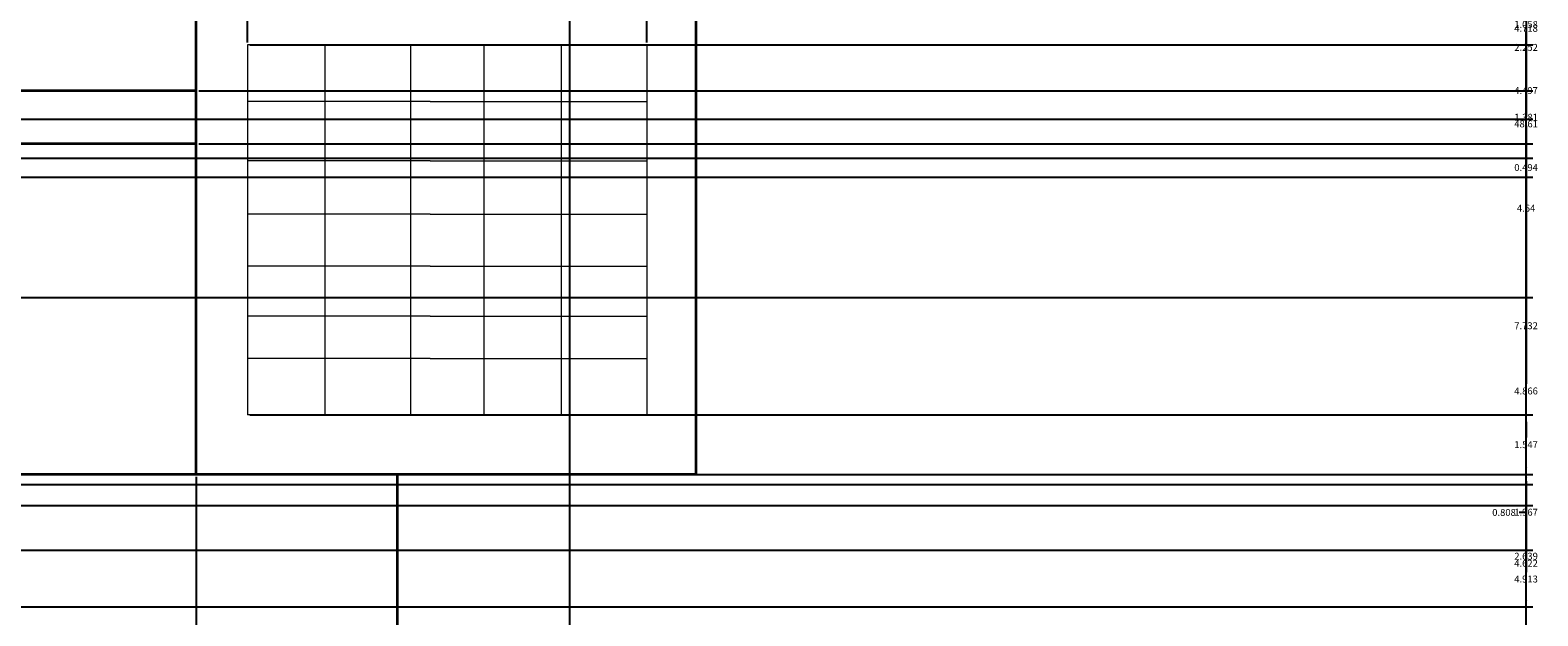
# Model space of a CAD drawing. Units: inches. Extents: x -10 to 130, y -32 to 34.
# Tile 20 of 22: x 90 to 130, y -10 to 5. Entities that reach past the tile are written whole.
import ezdxf

# ---------------------------------------------------------------- set-up
doc = ezdxf.new("R2010")
doc.units = ezdxf.units.IN
doc.header["$MEASUREMENT"] = 0
for name, color, linetype, lineweight in [('A-ANNO-DIMS', 2, 'Continuous', 18), ('A-ELEV', 7, 'Continuous', 35), ('A-GLAZ', 4, 'Continuous', 18)]:
    doc.layers.add(name, color=color, linetype=linetype, lineweight=lineweight)
doc.styles.get("Standard").update_dxf_attribs({"font": 'arial.ttf'})
doc.dimstyles.get("Standard").update_dxf_attribs({"dimtxt": 0.18, "dimasz": 0.18, "dimexe": 0.18, "dimexo": 0.0625, "dimgap": 0.09, "dimtad": 0, "dimtih": 1, "dimtoh": 1, "dimdec": 4, "dimzin": 0, "dimdsep": 46, "dimtxsty": 'Standard', "dimcen": 0.09, "dimadec": 0, "dimazin": 0, "dimtfac": 1, "dimtdec": 4, "dimtofl": 0, "dimtmove": 0, "dimatfit": 3, "dimfxl": 1, "dimtolj": 1, "dimtzin": 0, "dimarcsym": 0})

# ---------------------------------------------------------------- blocks, each defined once
blk = doc.blocks.new('*D2')
at = {"layer": 'A-ANNO-DIMS', "color": 0, "lineweight": -2, "transparency": 16777216}
for p, q in [((68.738, 27.199), (129.508, 27.199)), ((129.328, 27.019), (129.328, 3.074)), ((129.328, -21.234), (129.328, 2.71)), ((107.996, -21.414), (129.508, -21.414))]:
    blk.add_line(p, q, dxfattribs=at)
at = {"layer": 'A-ANNO-DIMS', "color": 0, "transparency": 16777216}
for points in [[(129.298, 27.019), (129.358, 27.019), (129.328, 27.199)], [(129.298, -21.234), (129.358, -21.234), (129.328, -21.414)]]:
    blk.add_solid(points, dxfattribs=at)
at = {"layer": 'Defpoints', "color": 0, "transparency": 16777216}
for p in [(68.676, 27.199), (129.328, 27.199), (107.933, -21.414)]:
    blk.add_point(p, dxfattribs=at)
at = {"layer": 'A-ANNO-DIMS', "color": 0, "transparency": 16777216, "insert": (129.328, 2.892), "char_height": 0.18, "attachment_point": 5}
blk.add_mtext('\\A1;48.61', dxfattribs=at)
blk = doc.blocks.new('*D66')
at = {"layer": 'A-ANNO-DIMS', "color": 0, "lineweight": -2, "transparency": 16777216}
for p, q in [((89.158, -16.844), (89.158, 33.879)), ((104.453, -13.219), (104.453, 33.879)), ((89.338, 33.699), (96.35, 33.699)), ((104.273, 33.699), (97.261, 33.699))]:
    blk.add_line(p, q, dxfattribs=at)
at = {"layer": 'A-ANNO-DIMS', "color": 0, "transparency": 16777216}
for points in [[(89.338, 33.729), (89.338, 33.669), (89.158, 33.699)], [(104.273, 33.729), (104.273, 33.669), (104.453, 33.699)]]:
    blk.add_solid(points, dxfattribs=at)
at = {"layer": 'Defpoints', "color": 0, "transparency": 16777216}
for p in [(104.453, 33.699), (104.453, -13.282), (89.158, -16.906)]:
    blk.add_point(p, dxfattribs=at)
at = {"layer": 'A-ANNO-DIMS', "color": 0, "transparency": 16777216, "insert": (96.805, 33.699), "char_height": 0.18, "attachment_point": 5}
blk.add_mtext('\\A1;15.295', dxfattribs=at)
blk = doc.blocks.new('*D76')
at = {"layer": 'A-ANNO-DIMS', "color": 0, "lineweight": -2, "transparency": 16777216}
for p, q in [((62.588, -6.485), (129.508, -6.485)), ((129.328, -6.665), (129.328, -8.76)), ((129.328, -11.218), (129.328, -9.123)), ((62.588, -11.398), (129.508, -11.398))]:
    blk.add_line(p, q, dxfattribs=at)
at = {"layer": 'A-ANNO-DIMS', "color": 0, "transparency": 16777216}
for points in [[(129.298, -6.665), (129.358, -6.665), (129.328, -6.485)], [(129.298, -11.218), (129.358, -11.218), (129.328, -11.398)]]:
    blk.add_solid(points, dxfattribs=at)
at = {"layer": 'Defpoints', "color": 0, "transparency": 16777216}
for p in [(62.526, -6.485), (129.328, -6.485), (62.526, -11.398)]:
    blk.add_point(p, dxfattribs=at)
at = {"layer": 'A-ANNO-DIMS', "color": 0, "transparency": 16777216, "insert": (129.328, -8.942), "char_height": 0.18, "attachment_point": 5}
blk.add_mtext('\\A1;4.913', dxfattribs=at)
blk = doc.blocks.new('*D77')
at = {"layer": 'A-ANNO-DIMS', "color": 0, "lineweight": -2, "transparency": 16777216}
for p, q in [((62.588, -1.618), (129.508, -1.618)), ((129.328, -1.798), (129.328, -3.87)), ((129.328, -6.305), (129.328, -4.234)), ((62.588, -6.485), (129.508, -6.485))]:
    blk.add_line(p, q, dxfattribs=at)
at = {"layer": 'A-ANNO-DIMS', "color": 0, "transparency": 16777216}
for points in [[(129.298, -1.798), (129.358, -1.798), (129.328, -1.618)], [(129.298, -6.305), (129.358, -6.305), (129.328, -6.485)]]:
    blk.add_solid(points, dxfattribs=at)
at = {"layer": 'Defpoints', "color": 0, "transparency": 16777216}
for p in [(62.526, -1.618), (129.328, -1.618), (62.526, -6.485)]:
    blk.add_point(p, dxfattribs=at)
at = {"layer": 'A-ANNO-DIMS', "color": 0, "transparency": 16777216, "insert": (129.328, -4.052), "char_height": 0.18, "attachment_point": 5}
blk.add_mtext('\\A1;4.866', dxfattribs=at)
blk = doc.blocks.new('*D78')
at = {"layer": 'A-ANNO-DIMS', "color": 0, "lineweight": -2, "transparency": 16777216}
for p, q in [((62.588, 3.018), (129.508, 3.018)), ((129.328, 2.838), (129.328, 0.882)), ((129.328, -1.438), (129.328, 0.518)), ((62.588, -1.618), (129.508, -1.618))]:
    blk.add_line(p, q, dxfattribs=at)
at = {"layer": 'A-ANNO-DIMS', "color": 0, "transparency": 16777216}
for points in [[(129.298, 2.838), (129.358, 2.838), (129.328, 3.018)], [(129.298, -1.438), (129.358, -1.438), (129.328, -1.618)]]:
    blk.add_solid(points, dxfattribs=at)
at = {"layer": 'Defpoints', "color": 0, "transparency": 16777216}
for p in [(62.526, 3.018), (129.328, 3.018), (62.526, -1.618)]:
    blk.add_point(p, dxfattribs=at)
at = {"layer": 'A-ANNO-DIMS', "color": 0, "transparency": 16777216, "insert": (129.328, 0.7), "char_height": 0.18, "attachment_point": 5}
blk.add_mtext('\\A1;4.64', dxfattribs=at)
blk = doc.blocks.new('*D79')
at = {"layer": 'A-ANNO-DIMS', "color": 0, "lineweight": -2, "transparency": 16777216}
for p, q in [((62.588, 7.736), (129.508, 7.736)), ((129.328, 7.556), (129.328, 5.559)), ((129.328, 3.198), (129.328, 5.195)), ((62.588, 3.018), (129.508, 3.018))]:
    blk.add_line(p, q, dxfattribs=at)
at = {"layer": 'A-ANNO-DIMS', "color": 0, "transparency": 16777216}
for points in [[(129.298, 7.556), (129.358, 7.556), (129.328, 7.736)], [(129.298, 3.198), (129.358, 3.198), (129.328, 3.018)]]:
    blk.add_solid(points, dxfattribs=at)
at = {"layer": 'Defpoints', "color": 0, "transparency": 16777216}
for p in [(62.526, 7.736), (129.328, 7.736), (62.526, 3.018)]:
    blk.add_point(p, dxfattribs=at)
at = {"layer": 'A-ANNO-DIMS', "color": 0, "transparency": 16777216, "insert": (129.328, 5.377), "char_height": 0.18, "attachment_point": 5}
blk.add_mtext('\\A1;4.718', dxfattribs=at)
blk = doc.blocks.new('*D153')
at = {"layer": 'A-ANNO-DIMS', "color": 0, "lineweight": -2, "transparency": 16777216}
for p, q in [((129.328, 2.185), (129.328, 2.365)), ((71.543, 2.005), (129.508, 2.005)), ((70.96, 1.511), (129.508, 1.511)), ((129.328, 1.331), (129.328, 1.151))]:
    blk.add_line(p, q, dxfattribs=at)
at = {"layer": 'A-ANNO-DIMS', "color": 0, "transparency": 16777216}
for points in [[(129.298, 2.185), (129.358, 2.185), (129.328, 2.005)], [(129.298, 1.331), (129.358, 1.331), (129.328, 1.511)]]:
    blk.add_solid(points, dxfattribs=at)
at = {"layer": 'Defpoints', "color": 0, "transparency": 16777216}
for p in [(71.48, 2.005), (70.898, 1.511), (129.328, 1.511)]:
    blk.add_point(p, dxfattribs=at)
at = {"layer": 'A-ANNO-DIMS', "color": 0, "transparency": 16777216, "insert": (129.328, 1.758), "char_height": 0.18, "attachment_point": 5}
blk.add_mtext('\\A1;0.494', dxfattribs=at)
blk = doc.blocks.new('*D154')
at = {"layer": 'A-ANNO-DIMS', "color": 0, "lineweight": -2, "transparency": 16777216}
for p, q in [((81.468, 6.007), (129.508, 6.007)), ((129.328, 5.827), (129.328, 3.941)), ((129.328, 1.691), (129.328, 3.577)), ((81.468, 1.511), (129.508, 1.511))]:
    blk.add_line(p, q, dxfattribs=at)
at = {"layer": 'A-ANNO-DIMS', "color": 0, "transparency": 16777216}
for points in [[(129.298, 5.827), (129.358, 5.827), (129.328, 6.007)], [(129.298, 1.691), (129.358, 1.691), (129.328, 1.511)]]:
    blk.add_solid(points, dxfattribs=at)
at = {"layer": 'Defpoints', "color": 0, "transparency": 16777216}
for p in [(81.405, 6.007), (129.328, 6.007), (81.405, 1.511)]:
    blk.add_point(p, dxfattribs=at)
at = {"layer": 'A-ANNO-DIMS', "color": 0, "transparency": 16777216, "insert": (129.328, 3.759), "char_height": 0.18, "attachment_point": 5}
blk.add_mtext('\\A1;4.497', dxfattribs=at)
blk = doc.blocks.new('*D159')
at = {"layer": 'A-ANNO-DIMS', "color": 0, "lineweight": -2, "transparency": 16777216}
for p, q in [((89.158, -6.284), (89.158, -28.129)), ((94.73, -6.284), (94.73, -28.129)), ((89.338, -27.949), (91.551, -27.949)), ((94.55, -27.949), (92.337, -27.949))]:
    blk.add_line(p, q, dxfattribs=at)
at = {"layer": 'A-ANNO-DIMS', "color": 0, "transparency": 16777216}
for points in [[(89.338, -27.919), (89.338, -27.979), (89.158, -27.949)], [(94.55, -27.919), (94.55, -27.979), (94.73, -27.949)]]:
    blk.add_solid(points, dxfattribs=at)
at = {"layer": 'Defpoints', "color": 0, "transparency": 16777216}
for p in [(89.158, -6.222), (94.73, -6.222), (94.73, -27.949)]:
    blk.add_point(p, dxfattribs=at)
at = {"layer": 'A-ANNO-DIMS', "color": 0, "transparency": 16777216, "insert": (91.944, -27.949), "char_height": 0.18, "attachment_point": 5}
blk.add_mtext('\\A1;5.572', dxfattribs=at)
blk = doc.blocks.new('*D160')
at = {"layer": 'A-ANNO-DIMS', "color": 0, "lineweight": -2, "transparency": 16777216}
for p, q in [((71.999, 1.511), (129.508, 1.511)), ((129.328, 1.331), (129.328, -2.174)), ((129.328, -6.042), (129.328, -2.538)), ((71.999, -6.222), (129.508, -6.222))]:
    blk.add_line(p, q, dxfattribs=at)
at = {"layer": 'A-ANNO-DIMS', "color": 0, "transparency": 16777216}
for points in [[(129.298, 1.331), (129.358, 1.331), (129.328, 1.511)], [(129.298, -6.042), (129.358, -6.042), (129.328, -6.222)]]:
    blk.add_solid(points, dxfattribs=at)
at = {"layer": 'Defpoints', "color": 0, "transparency": 16777216}
for p in [(71.937, 1.511), (71.937, -6.222), (129.328, -6.222)]:
    blk.add_point(p, dxfattribs=at)
at = {"layer": 'A-ANNO-DIMS', "color": 0, "transparency": 16777216, "insert": (129.328, -2.356), "char_height": 0.18, "attachment_point": 5}
blk.add_mtext('\\A1;7.732', dxfattribs=at)
blk = doc.blocks.new('*D161')
at = {"layer": 'A-ANNO-DIMS', "color": 0, "lineweight": -2, "transparency": 16777216}
for p, q in [((94.793, 6.007), (129.508, 6.007)), ((129.328, 5.827), (129.328, 5.064)), ((129.328, 3.936), (129.328, 4.7)), ((94.793, 3.756), (129.508, 3.756))]:
    blk.add_line(p, q, dxfattribs=at)
at = {"layer": 'A-ANNO-DIMS', "color": 0, "transparency": 16777216}
for points in [[(129.298, 5.827), (129.358, 5.827), (129.328, 6.007)], [(129.298, 3.936), (129.358, 3.936), (129.328, 3.756)]]:
    blk.add_solid(points, dxfattribs=at)
at = {"layer": 'Defpoints', "color": 0, "transparency": 16777216}
for p in [(94.73, 6.007), (94.73, 3.756), (129.328, 3.756)]:
    blk.add_point(p, dxfattribs=at)
at = {"layer": 'A-ANNO-DIMS', "color": 0, "transparency": 16777216, "insert": (129.328, 4.882), "char_height": 0.18, "attachment_point": 5}
blk.add_mtext('\\A1;2.252', dxfattribs=at)
blk = doc.blocks.new('*D162')
at = {"layer": 'A-ANNO-DIMS', "color": 0, "lineweight": -2, "transparency": 16777216}
for p, q in [((94.793, 3.756), (129.508, 3.756)), ((129.328, 3.576), (129.328, 3.247)), ((129.328, 2.555), (129.328, 2.883)), ((94.793, 2.375), (129.508, 2.375))]:
    blk.add_line(p, q, dxfattribs=at)
at = {"layer": 'A-ANNO-DIMS', "color": 0, "transparency": 16777216}
for points in [[(129.298, 3.576), (129.358, 3.576), (129.328, 3.756)], [(129.298, 2.555), (129.358, 2.555), (129.328, 2.375)]]:
    blk.add_solid(points, dxfattribs=at)
at = {"layer": 'Defpoints', "color": 0, "transparency": 16777216}
for p in [(94.73, 3.756), (94.73, 2.375), (129.328, 2.375)]:
    blk.add_point(p, dxfattribs=at)
at = {"layer": 'A-ANNO-DIMS', "color": 0, "transparency": 16777216, "insert": (129.328, 3.065), "char_height": 0.18, "attachment_point": 5}
blk.add_mtext('\\A1;1.381', dxfattribs=at)
blk = doc.blocks.new('*D163')
at = {"layer": 'A-ANNO-DIMS', "color": 0, "lineweight": -2, "transparency": 16777216}
for p, q in [((94.73, 6.07), (94.73, 33.879)), ((96.061, 5.012), (96.061, 33.879)), ((94.91, 33.699), (95.01, 33.699)), ((95.881, 33.699), (95.78, 33.699))]:
    blk.add_line(p, q, dxfattribs=at)
at = {"layer": 'A-ANNO-DIMS', "color": 0, "transparency": 16777216}
for points in [[(94.91, 33.729), (94.91, 33.669), (94.73, 33.699)], [(95.881, 33.729), (95.881, 33.669), (96.061, 33.699)]]:
    blk.add_solid(points, dxfattribs=at)
at = {"layer": 'Defpoints', "color": 0, "transparency": 16777216}
for p in [(96.061, 33.699), (94.73, 6.007), (96.061, 4.95)]:
    blk.add_point(p, dxfattribs=at)
at = {"layer": 'A-ANNO-DIMS', "color": 0, "transparency": 16777216, "insert": (95.395, 33.699), "char_height": 0.18, "attachment_point": 5}
blk.add_mtext('\\A1;1.330', dxfattribs=at)
blk = doc.blocks.new('*D164')
at = {"layer": 'A-ANNO-DIMS', "color": 0, "lineweight": -2, "transparency": 16777216}
for p, q in [((96.061, 5.012), (96.061, 33.879)), ((106.454, 5.012), (106.454, 33.879)), ((96.241, 33.699), (100.803, 33.699)), ((106.274, 33.699), (101.712, 33.699))]:
    blk.add_line(p, q, dxfattribs=at)
at = {"layer": 'A-ANNO-DIMS', "color": 0, "transparency": 16777216}
for points in [[(96.241, 33.729), (96.241, 33.669), (96.061, 33.699)], [(106.274, 33.729), (106.274, 33.669), (106.454, 33.699)]]:
    blk.add_solid(points, dxfattribs=at)
at = {"layer": 'Defpoints', "color": 0, "transparency": 16777216}
for p in [(106.454, 33.699), (96.061, 4.95), (106.454, 4.95)]:
    blk.add_point(p, dxfattribs=at)
at = {"layer": 'A-ANNO-DIMS', "color": 0, "transparency": 16777216, "insert": (101.257, 33.699), "char_height": 0.18, "attachment_point": 5}
blk.add_mtext('\\A1;10.394', dxfattribs=at)
blk = doc.blocks.new('*D165')
at = {"layer": 'A-ANNO-DIMS', "color": 0, "lineweight": -2, "transparency": 16777216}
for p, q in [((94.793, 6.007), (129.508, 6.007)), ((129.328, 5.827), (129.328, 5.66)), ((129.328, 5.13), (129.328, 5.297)), ((96.123, 4.95), (129.508, 4.95))]:
    blk.add_line(p, q, dxfattribs=at)
at = {"layer": 'A-ANNO-DIMS', "color": 0, "transparency": 16777216}
for points in [[(129.298, 5.827), (129.358, 5.827), (129.328, 6.007)], [(129.298, 5.13), (129.358, 5.13), (129.328, 4.95)]]:
    blk.add_solid(points, dxfattribs=at)
at = {"layer": 'Defpoints', "color": 0, "transparency": 16777216}
for p in [(94.73, 6.007), (129.328, 6.007), (96.061, 4.95)]:
    blk.add_point(p, dxfattribs=at)
at = {"layer": 'A-ANNO-DIMS', "color": 0, "transparency": 16777216, "insert": (129.328, 5.478), "char_height": 0.18, "attachment_point": 5}
blk.add_mtext('\\A1;1.058', dxfattribs=at)
blk = doc.blocks.new('*D166')
at = {"layer": 'A-ANNO-DIMS', "color": 0, "lineweight": -2, "transparency": 16777216}
for p, q in [((96.123, -4.675), (129.508, -4.675)), ((129.328, -4.855), (129.328, -5.266)), ((129.328, -6.042), (129.328, -5.63)), ((94.793, -6.222), (129.508, -6.222))]:
    blk.add_line(p, q, dxfattribs=at)
at = {"layer": 'A-ANNO-DIMS', "color": 0, "transparency": 16777216}
for points in [[(129.298, -4.855), (129.358, -4.855), (129.328, -4.675)], [(129.298, -6.042), (129.358, -6.042), (129.328, -6.222)]]:
    blk.add_solid(points, dxfattribs=at)
at = {"layer": 'Defpoints', "color": 0, "transparency": 16777216}
for p in [(96.061, -4.675), (94.73, -6.222), (129.328, -6.222)]:
    blk.add_point(p, dxfattribs=at)
at = {"layer": 'A-ANNO-DIMS', "color": 0, "transparency": 16777216, "insert": (129.328, -5.448), "char_height": 0.18, "attachment_point": 5}
blk.add_mtext('\\A1;1.547', dxfattribs=at)
blk = doc.blocks.new('*D168')
at = {"layer": 'A-ANNO-DIMS', "color": 0, "lineweight": -2, "transparency": 16777216}
for p, q in [((71.999, -6.222), (129.508, -6.222)), ((129.328, -6.402), (129.328, -7.024)), ((129.328, -8.009), (129.328, -7.387)), ((71.999, -8.189), (129.508, -8.189))]:
    blk.add_line(p, q, dxfattribs=at)
at = {"layer": 'A-ANNO-DIMS', "color": 0, "transparency": 16777216}
for points in [[(129.298, -6.402), (129.358, -6.402), (129.328, -6.222)], [(129.298, -8.009), (129.358, -8.009), (129.328, -8.189)]]:
    blk.add_solid(points, dxfattribs=at)
at = {"layer": 'Defpoints', "color": 0, "transparency": 16777216}
for p in [(71.937, -6.222), (71.937, -8.189), (129.328, -8.189)]:
    blk.add_point(p, dxfattribs=at)
at = {"layer": 'A-ANNO-DIMS', "color": 0, "transparency": 16777216, "insert": (129.328, -7.205), "char_height": 0.18, "attachment_point": 5}
blk.add_mtext('\\A1;1.967', dxfattribs=at)
blk = doc.blocks.new('*D171')
at = {"layer": 'A-ANNO-DIMS', "color": 0, "lineweight": -2, "transparency": 16777216}
for p, q in [((79.602, -7.03), (129.508, -7.03)), ((129.328, -7.21), (129.328, -8.167)), ((129.328, -9.489), (129.328, -8.531)), ((79.602, -9.669), (129.508, -9.669))]:
    blk.add_line(p, q, dxfattribs=at)
at = {"layer": 'A-ANNO-DIMS', "color": 0, "transparency": 16777216}
for points in [[(129.298, -7.21), (129.358, -7.21), (129.328, -7.03)], [(129.298, -9.489), (129.358, -9.489), (129.328, -9.669)]]:
    blk.add_solid(points, dxfattribs=at)
at = {"layer": 'Defpoints', "color": 0, "transparency": 16777216}
for p in [(79.539, -7.03), (79.539, -9.669), (129.328, -9.669)]:
    blk.add_point(p, dxfattribs=at)
at = {"layer": 'A-ANNO-DIMS', "color": 0, "transparency": 16777216, "insert": (129.328, -8.349), "char_height": 0.18, "attachment_point": 5}
blk.add_mtext('\\A1;2.639', dxfattribs=at)
blk = doc.blocks.new('*D172')
at = {"layer": 'A-ANNO-DIMS', "color": 0, "lineweight": -2, "transparency": 16777216}
for p, q in [((89.22, -6.222), (129.508, -6.222)), ((129.328, -6.402), (129.328, -6.85)), ((88.064, -7.03), (129.508, -7.03)), ((129.328, -7.03), (129.328, -7.21)), ((129.328, -7.21), (129.148, -7.21))]:
    blk.add_line(p, q, dxfattribs=at)
at = {"layer": 'A-ANNO-DIMS', "color": 0, "transparency": 16777216}
for points in [[(129.298, -6.402), (129.358, -6.402), (129.328, -6.222)], [(129.298, -6.85), (129.358, -6.85), (129.328, -7.03)]]:
    blk.add_solid(points, dxfattribs=at)
at = {"layer": 'Defpoints', "color": 0, "transparency": 16777216}
for p in [(89.158, -6.222), (88.002, -7.03), (129.328, -7.03)]:
    blk.add_point(p, dxfattribs=at)
at = {"layer": 'A-ANNO-DIMS', "color": 0, "transparency": 16777216, "insert": (128.754, -7.21), "char_height": 0.18, "attachment_point": 5}
blk.add_mtext('\\A1;0.808', dxfattribs=at)
blk = doc.blocks.new('*D174')
at = {"layer": 'A-ANNO-DIMS', "color": 0, "lineweight": -2, "transparency": 16777216}
for p, q in [((100.023, -6.222), (129.508, -6.222)), ((129.328, -6.402), (129.328, -8.351)), ((129.328, -10.663), (129.328, -8.715)), ((100.023, -10.843), (129.508, -10.843))]:
    blk.add_line(p, q, dxfattribs=at)
at = {"layer": 'A-ANNO-DIMS', "color": 0, "transparency": 16777216}
for points in [[(129.298, -6.402), (129.358, -6.402), (129.328, -6.222)], [(129.298, -10.663), (129.358, -10.663), (129.328, -10.843)]]:
    blk.add_solid(points, dxfattribs=at)
at = {"layer": 'Defpoints', "color": 0, "transparency": 16777216}
for p in [(99.96, -6.222), (99.96, -10.843), (129.328, -10.843)]:
    blk.add_point(p, dxfattribs=at)
at = {"layer": 'A-ANNO-DIMS', "color": 0, "transparency": 16777216, "insert": (129.328, -8.533), "char_height": 0.18, "attachment_point": 5}
blk.add_mtext('\\A1;4.622', dxfattribs=at)

msp = doc.modelspace()

# ---------------------------------------------------------------- linework, layer by layer
at = {"layer": 'A-ELEV'}
for p, q in [((94.7302, -6.2218), (94.7302, 6.0074)), ((107.7269, 6.0074), (107.7269, -6.2218)), ((94.7302, 3.7558), (89.1578, 3.7558)), ((94.7302, 2.375), (89.1578, 2.375)), ((94.7302, -6.2218), (89.1578, -6.2218)), ((107.7269, -6.2218), (94.7302, -6.2218)), ((99.9603, -6.2218), (99.9603, -10.8435))]:
    msp.add_line(p, q, dxfattribs=at)
at = {"layer": 'A-GLAZ'}
for p, q in [((98.6791, 4.9495), (96.0606, 4.9495)), ((96.0606, 4.9495), (96.0606, -4.6745)), ((100.8166, 4.9495), (97.276, 4.9495)), ((98.0756, 4.9495), (98.0756, -4.6745)), ((100.3029, 4.9495), (100.3029, -4.6745)), ((100.8166, 4.9495), (101.5409, 4.9495)), ((101.5409, 4.9495), (106.4542, 4.9495)), ((102.2119, 4.9495), (102.2119, -4.6745)), ((104.227, 4.9495), (104.227, -4.6745)), ((106.4542, 4.9495), (106.4542, -4.6745)), ((98.6791, 3.4745), (96.0606, 3.4745)), ((100.8166, 3.4745), (97.276, 3.4745)), ((100.8166, 3.4745), (101.5409, 3.4745)), ((101.5409, 3.4745), (106.4542, 3.4745)), ((98.6791, 1.9283), (96.0606, 1.9283)), ((100.8166, 1.9283), (97.276, 1.9283)), ((100.8166, 1.9283), (101.5409, 1.9283)), ((101.5409, 1.9283), (106.4542, 1.9283)), ((98.6791, 0.5449), (96.0606, 0.5449)), ((100.8166, 0.5449), (97.276, 0.5449)), ((100.8166, 0.5449), (101.5409, 0.5449)), ((101.5409, 0.5449), (106.4542, 0.5449)), ((98.6791, -0.809), (96.0606, -0.809)), ((100.8166, -0.809), (97.276, -0.809)), ((100.8166, -0.809), (101.5409, -0.809)), ((101.5409, -0.809), (106.4542, -0.809)), ((98.6791, -2.111), (96.0606, -2.111)), ((100.8166, -2.111), (97.276, -2.111)), ((100.8166, -2.111), (101.5409, -2.111)), ((101.5409, -2.111), (106.4542, -2.111)), ((98.6791, -3.2097), (96.0606, -3.2097)), ((100.8166, -3.2097), (97.276, -3.2097)), ((100.8166, -3.2097), (101.5409, -3.2097)), ((101.5409, -3.2097), (106.4542, -3.2097)), ((98.6791, -4.6745), (96.0606, -4.6745)), ((100.8166, -4.6745), (97.276, -4.6745)), ((100.8166, -4.6745), (101.5409, -4.6745)), ((101.5409, -4.6745), (106.4542, -4.6745))]:
    msp.add_line(p, q, dxfattribs=at)

# ---------------------------------------------------------------- dimensions: what is measured, and where the dimension line sits
at = {"layer": 'A-ANNO-DIMS'}
for base, p1, p2, picture, middle in [((104.4531, 33.6987), (89.1578, -16.9063), (104.4531, -13.2819), '*D66', (96.8055, 33.6987)), ((96.0606, 33.6987), (94.7302, 6.0074), (96.0606, 4.9495), '*D163', (95.3954, 33.6987)), ((106.4542, 33.6987), (96.0606, 4.9495), (106.4542, 4.9495), '*D164', (101.2574, 33.6987)), ((94.7302, -27.9493), (89.1578, -6.2218), (94.7302, -6.2218), '*D159', (91.944, -27.9493))]:
    dim = msp.add_linear_dim(base=base, p1=p1, p2=p2, dimstyle='Standard', override={"dimdec": 3, "dimlfac": 1, "dimrnd": 0, "dimzin": 0, "dimdsep": 46, "dimlunit": 2}, dxfattribs=at)
    dim.commit()
    dim.dimension.update_dxf_attribs({"geometry": picture, "text_midpoint": middle})
for base, p1, p2, override, picture, middle in [((129.3277, 27.1987), (107.9333, -21.4145), (68.6759, 27.1987), {"dimdec": 2, "dimlfac": 1, "dimrnd": 0, "dimzin": 0, "dimdsep": 46, "dimlunit": 2}, '*D2', (129.3277, 2.8921)), ((129.3277, 7.7364), (62.5256, 3.0181), (62.5256, 7.7364), {"dimdec": 3, "dimlfac": 1, "dimrnd": 0, "dimzin": 0, "dimdsep": 46, "dimlunit": 2}, '*D79', (129.3277, 5.3773)), ((129.3277, 6.0074), (81.4053, 1.5107), (81.4053, 6.0074), {"dimdec": 3, "dimlfac": 1, "dimrnd": 0, "dimzin": 0, "dimdsep": 46, "dimlunit": 2}, '*D154', (129.3277, 3.7591)), ((129.3277, 3.7558), (94.7302, 6.0074), (94.7302, 3.7558), {"dimdec": 3, "dimlfac": 1, "dimrnd": 0, "dimzin": 0, "dimdsep": 46, "dimlunit": 2}, '*D161', (129.3277, 4.8816)), ((129.3277, 6.0074), (96.0606, 4.9495), (94.7302, 6.0074), {"dimdec": 3, "dimlfac": 1, "dimrnd": 0, "dimzin": 0, "dimdsep": 46, "dimlunit": 2}, '*D165', (129.3277, 5.4785)), ((129.3277, 2.375), (94.7302, 3.7558), (94.7302, 2.375), {"dimdec": 3, "dimlfac": 1, "dimrnd": 0, "dimzin": 0, "dimdsep": 46, "dimlunit": 2}, '*D162', (129.3277, 3.0654)), ((129.3277, 3.0181), (62.5256, -1.6184), (62.5256, 3.0181), {"dimdec": 2, "dimlfac": 1, "dimrnd": 0, "dimzin": 0, "dimdsep": 46, "dimlunit": 2}, '*D78', (129.3277, 0.6998)), ((129.3277, 1.5107), (71.4801, 2.0049), (70.898, 1.5107), {"dimdec": 3, "dimlfac": 1, "dimrnd": 0, "dimzin": 0, "dimdsep": 46, "dimlunit": 2}, '*D153', (129.3277, 1.7578)), ((129.32767, -6.22179), (71.93671, 1.51067), (71.93671, -6.22179), {"dimdec": 3, "dimlfac": 1, "dimrnd": 0, "dimzin": 0, "dimdsep": 46, "dimlunit": 2}, '*D160', (129.32767, -2.35556)), ((129.32767, -1.61843), (62.52563, -6.48486), (62.52563, -1.61843), {"dimdec": 3, "dimlfac": 1, "dimrnd": 0, "dimzin": 0, "dimdsep": 46, "dimlunit": 2}, '*D77', (129.32767, -4.05165)), ((129.3277, -6.2218), (96.0606, -4.6745), (94.7302, -6.2218), {"dimdec": 3, "dimlfac": 1, "dimrnd": 0, "dimzin": 0, "dimdsep": 46, "dimlunit": 2}, '*D166', (129.3277, -5.4481)), ((129.3277, -8.1891), (71.9367, -6.2218), (71.9367, -8.1891), {"dimdec": 3, "dimlfac": 1, "dimrnd": 0, "dimzin": 0, "dimdsep": 46, "dimlunit": 2}, '*D168', (129.3277, -7.2054)), ((129.3277, -7.0301), (89.1578, -6.2218), (88.0017, -7.0301), {"dimdec": 3, "dimlfac": 1, "dimrnd": 0, "dimzin": 0, "dimdsep": 46, "dimlunit": 2}, '*D172', (128.7538, -7.2101)), ((129.3277, -10.8435), (99.9603, -6.2218), (99.9603, -10.8435), {"dimdec": 3, "dimlfac": 1, "dimrnd": 0, "dimzin": 0, "dimdsep": 46, "dimlunit": 2}, '*D174', (129.3277, -8.5326)), ((129.3277, -6.4849), (62.5256, -11.3982), (62.5256, -6.4849), {"dimdec": 3, "dimlfac": 1, "dimrnd": 0, "dimzin": 0, "dimdsep": 46, "dimlunit": 2}, '*D76', (129.3277, -8.9415)), ((129.3277, -9.6688), (79.5394, -7.0301), (79.5394, -9.6688), {"dimdec": 3, "dimlfac": 1, "dimrnd": 0, "dimzin": 0, "dimdsep": 46, "dimlunit": 2}, '*D171', (129.3277, -8.3494))]:
    dim = msp.add_linear_dim(base=base, p1=p1, p2=p2, angle=90, dimstyle='Standard', override=override, dxfattribs=at)
    dim.commit()
    dim.dimension.update_dxf_attribs({"geometry": picture, "text_midpoint": middle})

doc.saveas('drawing.dxf')
